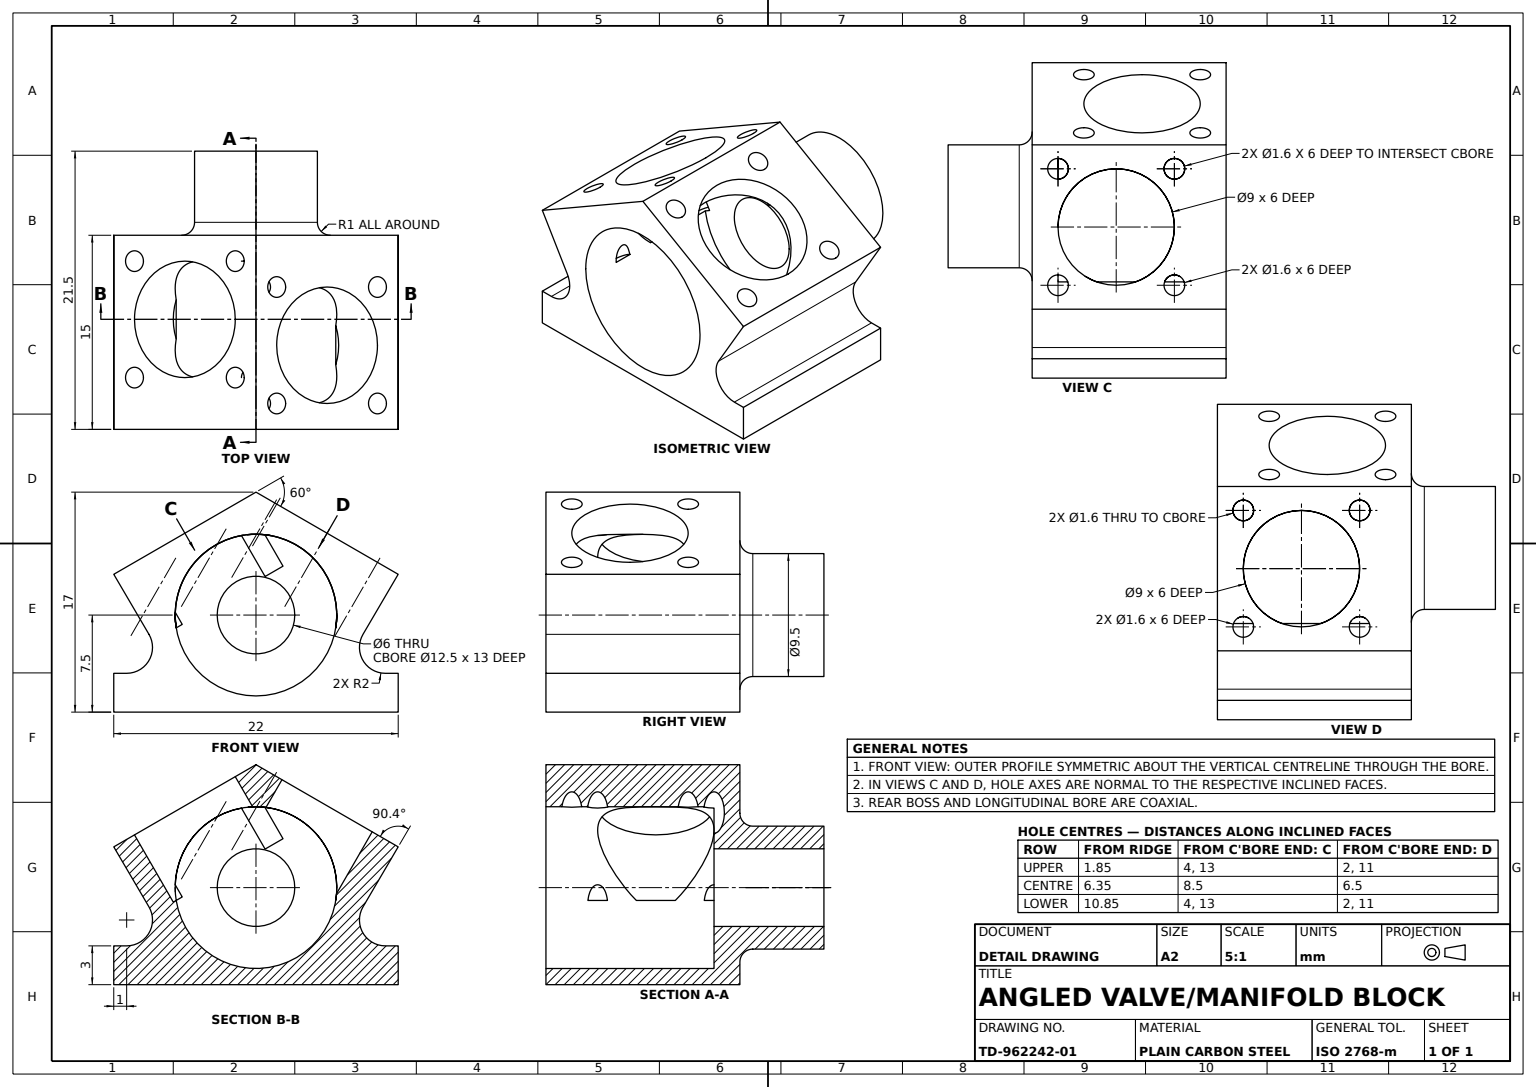
from build123d import *

# Parameters (mm, degrees)
HOUSING_PROFILE_SKETCH_R  = 6.25
HOUSING_BODY_DEPTH        = 15
CYLINDRICAL_BOSS_SKETCH_R = 4.75
CYLINDRICAL_BOSS_DEPTH    = 6.5
BOSS_START                = -2
BOSS_COLLAR_SKETCH_R      = 6.25
BOSS_COLLAR_DEPTH         = 2
THROUGH_BORE_SKETCH_R     = 3
THROUGH_BORE_DEPTH        = 43
FACE_HOLES_A_SKETCH_R     = 4.5
FACE_HOLES_A_SKETCH_R_2   = 0.8
FACE_HOLES_A_DEPTH        = 6
FACE_HOLES_B_SKETCH_R     = 4.5
FACE_HOLES_B_SKETCH_R_2   = 0.8
FACE_HOLES_B_DEPTH        = 6
EDGE_FILLET_R1_R          = 1


with BuildPart() as part:
    # Housing Profile Sketch → Housing Body (new body)
    with BuildSketch(Plane.XY):
        with BuildLine():
            Line((0, 17), (-10.998522628, 10.65))
            Line((-10.998522628, 10.65), (-8.277038378, 6.010719954))
            ThreePointArc((-8.277038378, 6.010719954), (-8.26662318, 4.004754709), (-10.002124982, 2.998753448))
            Line((-10.002124982, 2.998753448), (-11, 2.998753448))
            Line((-11, 2.998753448), (-11, 0))
            Line((-11, 0), (-10.002124982, 0))
            Line((-10.002124982, 0), (10.002124982, 0))
            Line((10.002124982, 0), (11, 0))
            Line((11, 0), (11, 2.998753448))
            Line((11, 2.998753448), (10.002124982, 2.998753448))
            ThreePointArc((10.002124982, 2.998753448), (8.26662318, 4.004754709), (8.277038378, 6.010719954))
            Line((8.277038378, 6.010719954), (10.998522628, 10.65))
            Line((10.998522628, 10.65), (0, 17))
        make_face()
        with Locations((0, 7.5)):
            Circle(HOUSING_PROFILE_SKETCH_R, mode=Mode.SUBTRACT)
    extrude(amount=-HOUSING_BODY_DEPTH)



with BuildPart() as body_2:
    # Cylindrical Boss Sketch → Cylindrical Boss (new body)
    with BuildSketch(Plane(origin=(0, 0, -15), x_dir=(-1, 0, 0), z_dir=(0, 0, -1))):
        with Locations(Location((0, 7.5, 0), (0, 0, 180))):
            Circle(CYLINDRICAL_BOSS_SKETCH_R)
    extrude(amount=CYLINDRICAL_BOSS_DEPTH)


with BuildPart() as part_1:
    add(part.part)

    add(body_2.part)  # Boss Collar merges body 2
    # Boss Collar Sketch → Boss Collar (add)
    with BuildSketch(Plane(origin=(0, 0, -15), x_dir=(-1, 0, 0), z_dir=(0, 0, -1)).offset(BOSS_START)):
        with Locations(Location((0, 7.5, 0), (0, 0, 180))):
            Circle(BOSS_COLLAR_SKETCH_R)
    extrude(amount=BOSS_COLLAR_DEPTH)

    # Through Bore Sketch → Through Bore (cut)
    with BuildSketch(Plane(origin=(0, 0, -21.5), x_dir=(-1, 0, 0), z_dir=(0, 0, -1))):
        with Locations((0, 7.5)):
            Circle(THROUGH_BORE_SKETCH_R)
    extrude(amount=-THROUGH_BORE_DEPTH, mode=Mode.SUBTRACT)

    # Face Holes A Sketch → Face Holes A (cut)
    with BuildSketch(Plane(origin=(7.361215932, 12.75, 0), x_dir=(0.8660254037844394, -0.4999999999999988, 0), z_dir=(0.4999999999999988, 0.8660254037844394, 0))):
        with Locations(Location((-2.15, 6.5, 0), (0, 0, 180))):
            Circle(FACE_HOLES_A_SKETCH_R)
        with Locations(Location((2.35, 11, 0), (0, 0, 180))):
            Circle(FACE_HOLES_A_SKETCH_R_2)
        with Locations(Location((2.35, 2, 0), (0, 0, 149.224237469))):
            Circle(FACE_HOLES_A_SKETCH_R_2)
        with Locations(Location((-6.65, 2, 0), (0, 0, 180))):
            Circle(FACE_HOLES_A_SKETCH_R_2)
        with Locations(Location((-6.65, 11, 0), (0, 0, 180))):
            Circle(FACE_HOLES_A_SKETCH_R_2)
    extrude(amount=-FACE_HOLES_A_DEPTH, mode=Mode.SUBTRACT)

    # Face Holes B Sketch → Face Holes B (cut)
    with BuildSketch(Plane(origin=(-7.361215932, 12.75, 0), x_dir=(0.8660254037844403, 0.4999999999999971, 0), z_dir=(-0.49999999999999717, 0.8660254037844404, 0))):
        with Locations(Location((2.15, 8.5, 0), (0, 0, 180))):
            Circle(FACE_HOLES_B_SKETCH_R)
        with Locations(Location((-2.35, 13, 0), (0, 0, 180))):
            Circle(FACE_HOLES_B_SKETCH_R_2)
        with Locations((6.65, 13)):
            Circle(FACE_HOLES_B_SKETCH_R_2)
        with Locations(Location((6.65, 4, 0), (0, 0, 180))):
            Circle(FACE_HOLES_B_SKETCH_R_2)
        with Locations(Location((-2.35, 4, 0), (0, 0, 71.010406817))):
            Circle(FACE_HOLES_B_SKETCH_R_2)
    extrude(amount=-FACE_HOLES_B_DEPTH, mode=Mode.SUBTRACT)

    # Edge Fillet R1
    edge_fillet_r1_edges = [part_1.edges().sort_by_distance(p)[0] for p in [
        (-4.75, 7.5, -15),
    ]]
    fillet(edge_fillet_r1_edges, radius=EDGE_FILLET_R1_R)


solid = part_1.part
